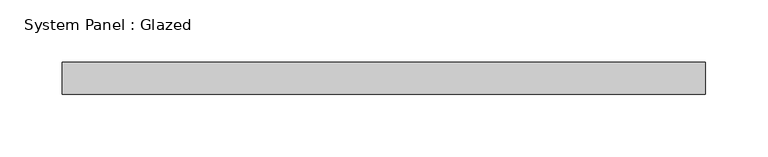
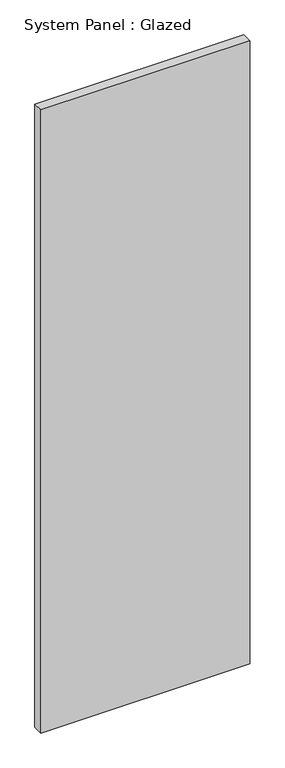
"""IFC4 building model written with IfcOpenShell, lengths in millimetres: plate geometry, System Panel : Glazed."""

from ifc_helpers import new_model, si_unit, origin, origin_with_axes, place, context, project, spatial, polyline, outline, extrude, source, transform, mapped, element, save


def system_panel_glazed_cb3ffd69(model_context):
    return source(origin(), model_context, "Body", "SweptSolid", [
        extrude(outline(polyline([(257.6030168, 19.05), (-257.6030168, 19.05), (-257.6030168, 44.45), (257.6030168, 44.45), (257.6030168, 19.05)])), origin_with_axes(), (0.0, 0.0, 1.0), 1625.6),
    ])


if __name__ == "__main__":
    model = new_model("IFC4")
    model_context = context("Model", 3, world=origin())
    ifc_project = project(units=[si_unit("LENGTHUNIT", "METRE", prefix="MILLI")], contexts=[model_context])
    site = spatial("IfcSite", under=ifc_project)
    building = spatial("IfcBuilding", under=site)
    placement = place(None, origin())
    system_panel_glazed_shape = system_panel_glazed_cb3ffd69(model_context)
    element("IfcPlate", 1, ObjectType="System Panel : Glazed", at=placement, inside=building, context=model_context, shape_type="MappedRepresentation", body=[
        mapped(system_panel_glazed_shape, transform((0.0, 0.0, 0.0), x_axis=(1.0, 0.0, 0.0), y_axis=(0.0, 1.0, 0.0), z_axis=(0.0, 0.0, 1.0))),
    ])
    save(model, "model.ifc")

# Revit data of these elements
# Type "System Panel : Glazed"
#   Construction Type Id = "GSP4R"
#   Analytic Construction = "1/8 in Pilkington single glazing"
#   Visual Light Transmittance = 0.9
#   Solar Heat Gain Coefficient = 0.86
#   Heat Transfer Coefficient (U) = 1.18115 BTU/(h·ft²·°F)
# Element 1 (IfcPlate, "System Panel : Glazed")
#   Materials on its faces: "Glass"
# Materials
#   "Glass": class "Glass", colour RGB 0 128 192, transparency 0.75, Description = "Soda Lime Glass", Cost = 0
